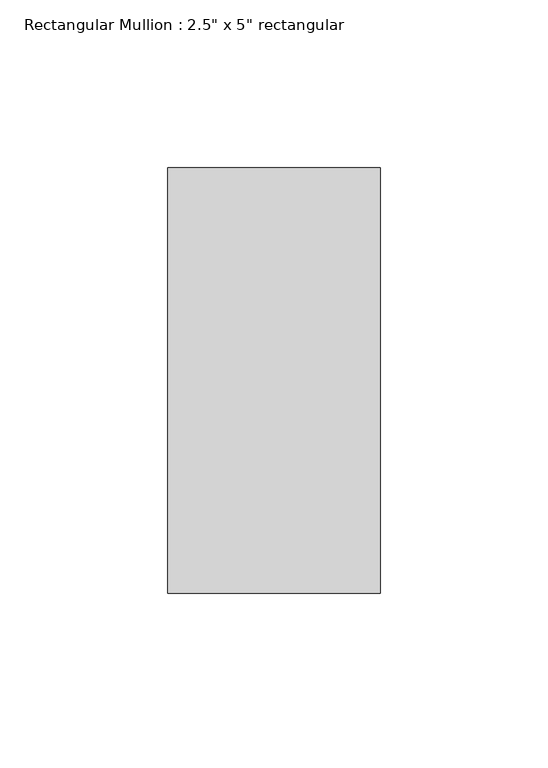
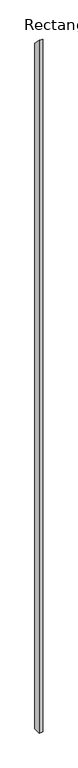
"""IFC4 building model written with IfcOpenShell, lengths in millimetres: member geometry."""

from ifc_helpers import new_model, si_unit, frame, origin, place, context, project, spatial, polyline, outline, extrude, source, transform, mapped, element, save


def member_60525e8a(model_context):
    return source(origin(), model_context, "Body", "SweptSolid", [
        extrude(outline(polyline([(-63.5, 63.5), (63.5, -63.5), (63.5, -12555.5552746), (-63.5, -12555.5552746), (-63.5, 63.5)])), frame((-63.5, 0.0, 0.0), z_axis=(1.0, 0.0, 0.0), x_axis=(0.0, 1.0, 0.0)), (0.0, 0.0, 1.0), 63.5),
    ])


if __name__ == "__main__":
    model = new_model("IFC4")
    model_context = context("Model", 3, world=origin())
    ifc_project = project(units=[si_unit("LENGTHUNIT", "METRE", prefix="MILLI")], contexts=[model_context])
    site = spatial("IfcSite", under=ifc_project)
    building = spatial("IfcBuilding", under=site)
    placement = place(None, origin())
    member_shape = member_60525e8a(model_context)
    element("IfcMember", 1, ObjectType="Rectangular Mullion : 2.5\" x 5\" rectangular", at=placement, inside=building, context=model_context, shape_type="MappedRepresentation", body=[
        mapped(member_shape, transform((0.0, 0.0, 0.0), x_axis=(1.0, 0.0, 0.0), y_axis=(0.0, 1.0, 0.0), z_axis=(0.0, 0.0, 1.0))),
    ])
    save(model, "model.ifc")

# Revit data of these elements
# Type "Rectangular Mullion : 2.5\" x 5\" rectangular"
#   built-in parameter 1007304 = 0.416667 (stored number, unit not read)
#   built-in parameter 1007301 = 0.104167 (stored number, unit not read)
#   built-in parameter 1007300 = 0.104167 (stored number, unit not read)
# Element 1 (IfcMember, "Rectangular Mullion : 2.5\" x 5\" rectangular")
#   Materials on its faces: "Aluminum"
# Materials
#   "Aluminum": class "Metal", colour RGB 247 247 247, transparency 0, Description = "Aluminum 6061", Cost = 0
